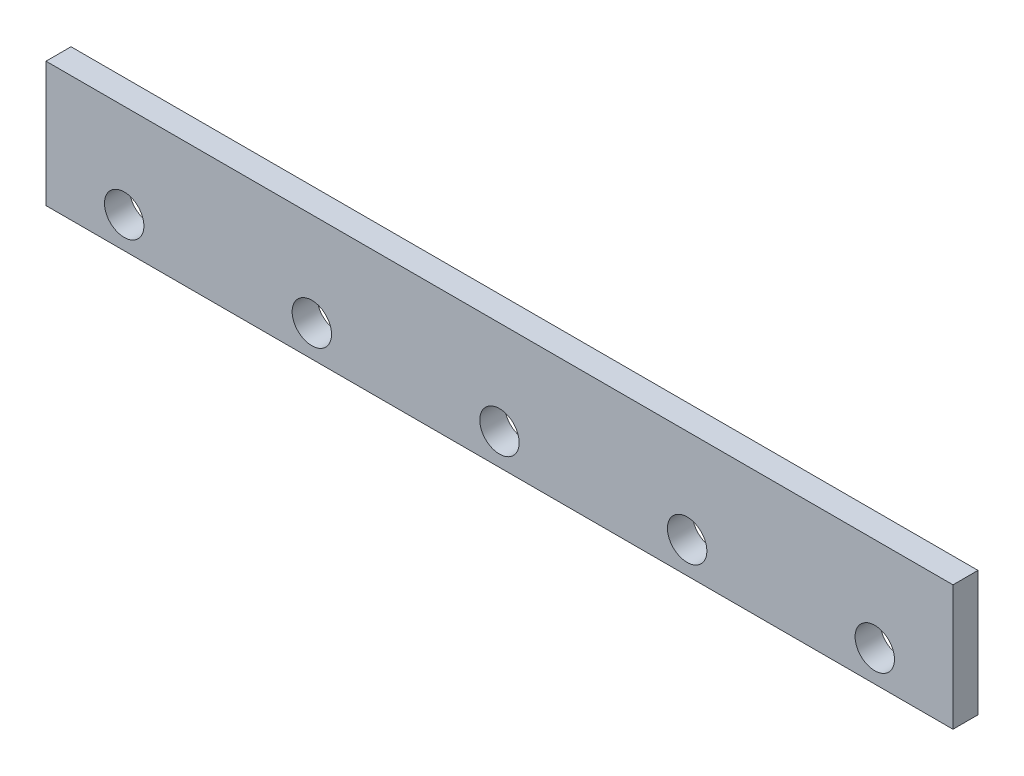
ISO-10303-21;
HEADER;
FILE_DESCRIPTION(('STEP AP214'),'2;1');
FILE_NAME('part.step','',(''),(''),'','','');
FILE_SCHEMA(('AUTOMOTIVE_DESIGN { 1 0 10303 214 1 1 1 1 }'));
ENDSEC;
DATA;
#1=APPLICATION_CONTEXT('core data for automotive mechanical design processes');
#2=APPLICATION_PROTOCOL_DEFINITION('international standard','automotive_design',2000,#1);
#3=PRODUCT_CONTEXT('',#1,'mechanical');
#4=PRODUCT('Part','Part','',(#3));
#5=PRODUCT_RELATED_PRODUCT_CATEGORY('part','',(#4));
#6=PRODUCT_DEFINITION_FORMATION('','',#4);
#7=PRODUCT_DEFINITION_CONTEXT('part definition',#1,'design');
#8=PRODUCT_DEFINITION('design','',#6,#7);
#9=PRODUCT_DEFINITION_SHAPE('','',#8);
#10=(LENGTH_UNIT() NAMED_UNIT(*) SI_UNIT(.MILLI.,.METRE.));
#11=(NAMED_UNIT(*) PLANE_ANGLE_UNIT() SI_UNIT($,.RADIAN.));
#12=(NAMED_UNIT(*) SI_UNIT($,.STERADIAN.) SOLID_ANGLE_UNIT());
#13=UNCERTAINTY_MEASURE_WITH_UNIT(LENGTH_MEASURE(1.E-05),#10,'distance_accuracy_value','');
#14=(GEOMETRIC_REPRESENTATION_CONTEXT(3) GLOBAL_UNCERTAINTY_ASSIGNED_CONTEXT((#13)) GLOBAL_UNIT_ASSIGNED_CONTEXT((#10,
#11,#12)) REPRESENTATION_CONTEXT('',''));
#15=CARTESIAN_POINT('',(0.,0.,0.));
#16=DIRECTION('',(0.,0.,1.));
#17=DIRECTION('',(1.,0.,0.));
#18=AXIS2_PLACEMENT_3D('',#15,#16,#17);
#19=CARTESIAN_POINT('',(290.,40.,16.));
#20=DIRECTION('',(-1.,0.,0.));
#21=DIRECTION('',(0.,0.,1.));
#22=AXIS2_PLACEMENT_3D('',#19,#20,#21);
#23=PLANE('',#22);
#24=DIRECTION('',(0.,1.,0.));
#25=VECTOR('',#24,1.);
#26=CARTESIAN_POINT('',(290.,40.,0.));
#27=LINE('',#26,#25);
#28=CARTESIAN_POINT('',(290.,-40.,0.));
#29=VERTEX_POINT('',#28);
#30=CARTESIAN_POINT('',(290.,40.,0.));
#31=VERTEX_POINT('',#30);
#32=EDGE_CURVE('E102',#29,#31,#27,.T.);
#33=ORIENTED_EDGE('',*,*,#32,.T.);
#34=DIRECTION('',(0.,0.,-1.));
#35=VECTOR('',#34,1.);
#36=CARTESIAN_POINT('',(290.,40.,16.));
#37=LINE('',#36,#35);
#38=CARTESIAN_POINT('',(290.,40.,16.));
#39=VERTEX_POINT('',#38);
#40=EDGE_CURVE('E11',#39,#31,#37,.T.);
#41=ORIENTED_EDGE('',*,*,#40,.F.);
#42=DIRECTION('',(0.,1.,0.));
#43=VECTOR('',#42,1.);
#44=CARTESIAN_POINT('',(290.,40.,16.));
#45=LINE('',#44,#43);
#46=CARTESIAN_POINT('',(290.,-40.,16.));
#47=VERTEX_POINT('',#46);
#48=EDGE_CURVE('E95',#47,#39,#45,.T.);
#49=ORIENTED_EDGE('',*,*,#48,.F.);
#50=DIRECTION('',(0.,0.,-1.));
#51=VECTOR('',#50,1.);
#52=CARTESIAN_POINT('',(290.,-40.,16.));
#53=LINE('',#52,#51);
#54=EDGE_CURVE('E103',#47,#29,#53,.T.);
#55=ORIENTED_EDGE('',*,*,#54,.T.);
#56=EDGE_LOOP('',(#33,#41,#49,#55));
#57=FACE_BOUND('',#56,.T.);
#58=ADVANCED_FACE('F39',(#57),#23,.F.);
#59=CARTESIAN_POINT('',(-290.,40.,16.));
#60=DIRECTION('',(0.,-1.,0.));
#61=DIRECTION('',(0.,0.,-1.));
#62=AXIS2_PLACEMENT_3D('',#59,#60,#61);
#63=PLANE('',#62);
#64=DIRECTION('',(-1.,0.,0.));
#65=VECTOR('',#64,1.);
#66=CARTESIAN_POINT('',(-290.,40.,0.));
#67=LINE('',#66,#65);
#68=CARTESIAN_POINT('',(-290.,40.,0.));
#69=VERTEX_POINT('',#68);
#70=EDGE_CURVE('E98',#31,#69,#67,.T.);
#71=ORIENTED_EDGE('',*,*,#70,.T.);
#72=DIRECTION('',(0.,0.,-1.));
#73=VECTOR('',#72,1.);
#74=CARTESIAN_POINT('',(-290.,40.,16.));
#75=LINE('',#74,#73);
#76=CARTESIAN_POINT('',(-290.,40.,16.));
#77=VERTEX_POINT('',#76);
#78=EDGE_CURVE('E48',#77,#69,#75,.T.);
#79=ORIENTED_EDGE('',*,*,#78,.F.);
#80=DIRECTION('',(-1.,0.,0.));
#81=VECTOR('',#80,1.);
#82=CARTESIAN_POINT('',(-290.,40.,16.));
#83=LINE('',#82,#81);
#84=EDGE_CURVE('E90',#39,#77,#83,.T.);
#85=ORIENTED_EDGE('',*,*,#84,.F.);
#86=ORIENTED_EDGE('',*,*,#40,.T.);
#87=EDGE_LOOP('',(#71,#79,#85,#86));
#88=FACE_BOUND('',#87,.T.);
#89=ADVANCED_FACE('F94',(#88),#63,.F.);
#90=CARTESIAN_POINT('',(-290.,40.,16.));
#91=DIRECTION('',(1.,0.,0.));
#92=DIRECTION('',(0.,0.,-1.));
#93=AXIS2_PLACEMENT_3D('',#90,#91,#92);
#94=PLANE('',#93);
#95=DIRECTION('',(0.,-1.,0.));
#96=VECTOR('',#95,1.);
#97=CARTESIAN_POINT('',(-290.,40.,0.));
#98=LINE('',#97,#96);
#99=CARTESIAN_POINT('',(-290.,-40.,0.));
#100=VERTEX_POINT('',#99);
#101=EDGE_CURVE('E72',#69,#100,#98,.T.);
#102=ORIENTED_EDGE('',*,*,#101,.T.);
#103=DIRECTION('',(0.,0.,-1.));
#104=VECTOR('',#103,1.);
#105=CARTESIAN_POINT('',(-290.,-40.,16.));
#106=LINE('',#105,#104);
#107=CARTESIAN_POINT('',(-290.,-40.,16.));
#108=VERTEX_POINT('',#107);
#109=EDGE_CURVE('E97',#108,#100,#106,.T.);
#110=ORIENTED_EDGE('',*,*,#109,.F.);
#111=DIRECTION('',(0.,-1.,0.));
#112=VECTOR('',#111,1.);
#113=CARTESIAN_POINT('',(-290.,40.,16.));
#114=LINE('',#113,#112);
#115=EDGE_CURVE('E89',#77,#108,#114,.T.);
#116=ORIENTED_EDGE('',*,*,#115,.F.);
#117=ORIENTED_EDGE('',*,*,#78,.T.);
#118=EDGE_LOOP('',(#102,#110,#116,#117));
#119=FACE_BOUND('',#118,.T.);
#120=ADVANCED_FACE('F100',(#119),#94,.F.);
#121=CARTESIAN_POINT('',(-290.,-40.,16.));
#122=DIRECTION('',(0.,1.,0.));
#123=DIRECTION('',(0.,0.,1.));
#124=AXIS2_PLACEMENT_3D('',#121,#122,#123);
#125=PLANE('',#124);
#126=DIRECTION('',(1.,0.,0.));
#127=VECTOR('',#126,1.);
#128=CARTESIAN_POINT('',(-290.,-40.,0.));
#129=LINE('',#128,#127);
#130=EDGE_CURVE('E78',#100,#29,#129,.T.);
#131=ORIENTED_EDGE('',*,*,#130,.T.);
#132=ORIENTED_EDGE('',*,*,#54,.F.);
#133=DIRECTION('',(1.,0.,0.));
#134=VECTOR('',#133,1.);
#135=CARTESIAN_POINT('',(-290.,-40.,16.));
#136=LINE('',#135,#134);
#137=EDGE_CURVE('E60',#108,#47,#136,.T.);
#138=ORIENTED_EDGE('',*,*,#137,.F.);
#139=ORIENTED_EDGE('',*,*,#109,.T.);
#140=EDGE_LOOP('',(#131,#132,#138,#139));
#141=FACE_BOUND('',#140,.T.);
#142=ADVANCED_FACE('F159',(#141),#125,.F.);
#143=CARTESIAN_POINT('',(0.,0.,16.));
#144=DIRECTION('',(0.,0.,1.));
#145=DIRECTION('',(1.,0.,0.));
#146=AXIS2_PLACEMENT_3D('',#143,#144,#145);
#147=PLANE('',#146);
#148=CARTESIAN_POINT('',(-240.,-20.,16.));
#149=DIRECTION('',(0.,0.,1.));
#150=DIRECTION('',(1.,0.,0.));
#151=AXIS2_PLACEMENT_3D('',#148,#149,#150);
#152=CIRCLE('',#151,12.6);
#153=CARTESIAN_POINT('',(-227.4,-20.,16.));
#154=VERTEX_POINT('',#153);
#155=EDGE_CURVE('E120',#154,#154,#152,.T.);
#156=ORIENTED_EDGE('',*,*,#155,.F.);
#157=EDGE_LOOP('',(#156));
#158=FACE_BOUND('',#157,.T.);
#159=CARTESIAN_POINT('',(-120.,-20.,16.));
#160=DIRECTION('',(0.,0.,1.));
#161=DIRECTION('',(1.,0.,0.));
#162=AXIS2_PLACEMENT_3D('',#159,#160,#161);
#163=CIRCLE('',#162,12.6);
#164=CARTESIAN_POINT('',(-107.4,-20.,16.));
#165=VERTEX_POINT('',#164);
#166=EDGE_CURVE('E236',#165,#165,#163,.T.);
#167=ORIENTED_EDGE('',*,*,#166,.F.);
#168=EDGE_LOOP('',(#167));
#169=FACE_BOUND('',#168,.T.);
#170=CARTESIAN_POINT('',(1.11022302462516E-13,-20.,16.));
#171=DIRECTION('',(0.,0.,1.));
#172=DIRECTION('',(1.,0.,0.));
#173=AXIS2_PLACEMENT_3D('',#170,#171,#172);
#174=CIRCLE('',#173,12.6);
#175=CARTESIAN_POINT('',(12.6000000000001,-20.,16.));
#176=VERTEX_POINT('',#175);
#177=EDGE_CURVE('E228',#176,#176,#174,.T.);
#178=ORIENTED_EDGE('',*,*,#177,.F.);
#179=EDGE_LOOP('',(#178));
#180=FACE_BOUND('',#179,.T.);
#181=CARTESIAN_POINT('',(120.,-20.,16.));
#182=DIRECTION('',(0.,0.,1.));
#183=DIRECTION('',(1.,0.,0.));
#184=AXIS2_PLACEMENT_3D('',#181,#182,#183);
#185=CIRCLE('',#184,12.6);
#186=CARTESIAN_POINT('',(132.6,-20.,16.));
#187=VERTEX_POINT('',#186);
#188=EDGE_CURVE('E240',#187,#187,#185,.T.);
#189=ORIENTED_EDGE('',*,*,#188,.F.);
#190=EDGE_LOOP('',(#189));
#191=FACE_BOUND('',#190,.T.);
#192=CARTESIAN_POINT('',(240.,-20.,16.));
#193=DIRECTION('',(0.,0.,1.));
#194=DIRECTION('',(1.,0.,0.));
#195=AXIS2_PLACEMENT_3D('',#192,#193,#194);
#196=CIRCLE('',#195,12.6);
#197=CARTESIAN_POINT('',(252.6,-20.,16.));
#198=VERTEX_POINT('',#197);
#199=EDGE_CURVE('E245',#198,#198,#196,.T.);
#200=ORIENTED_EDGE('',*,*,#199,.F.);
#201=EDGE_LOOP('',(#200));
#202=FACE_BOUND('',#201,.T.);
#203=ORIENTED_EDGE('',*,*,#48,.T.);
#204=ORIENTED_EDGE('',*,*,#84,.T.);
#205=ORIENTED_EDGE('',*,*,#115,.T.);
#206=ORIENTED_EDGE('',*,*,#137,.T.);
#207=EDGE_LOOP('',(#203,#204,#205,#206));
#208=FACE_BOUND('',#207,.T.);
#209=ADVANCED_FACE('F88',(#158,#169,#180,#191,#202,#208),#147,.T.);
#210=CARTESIAN_POINT('',(0.,0.,0.));
#211=DIRECTION('',(0.,0.,1.));
#212=DIRECTION('',(1.,0.,0.));
#213=AXIS2_PLACEMENT_3D('',#210,#211,#212);
#214=PLANE('',#213);
#215=CARTESIAN_POINT('',(-240.,-20.,0.));
#216=DIRECTION('',(0.,0.,1.));
#217=DIRECTION('',(1.,0.,0.));
#218=AXIS2_PLACEMENT_3D('',#215,#216,#217);
#219=CIRCLE('',#218,12.6);
#220=CARTESIAN_POINT('',(-227.4,-20.,0.));
#221=VERTEX_POINT('',#220);
#222=EDGE_CURVE('E45',#221,#221,#219,.T.);
#223=ORIENTED_EDGE('',*,*,#222,.T.);
#224=EDGE_LOOP('',(#223));
#225=FACE_BOUND('',#224,.T.);
#226=CARTESIAN_POINT('',(-120.,-20.,0.));
#227=DIRECTION('',(0.,0.,1.));
#228=DIRECTION('',(1.,0.,0.));
#229=AXIS2_PLACEMENT_3D('',#226,#227,#228);
#230=CIRCLE('',#229,12.6);
#231=CARTESIAN_POINT('',(-107.4,-20.,0.));
#232=VERTEX_POINT('',#231);
#233=EDGE_CURVE('E125',#232,#232,#230,.T.);
#234=ORIENTED_EDGE('',*,*,#233,.T.);
#235=EDGE_LOOP('',(#234));
#236=FACE_BOUND('',#235,.T.);
#237=CARTESIAN_POINT('',(1.11022302462516E-13,-20.,0.));
#238=DIRECTION('',(0.,0.,1.));
#239=DIRECTION('',(1.,0.,0.));
#240=AXIS2_PLACEMENT_3D('',#237,#238,#239);
#241=CIRCLE('',#240,12.6);
#242=CARTESIAN_POINT('',(12.6000000000001,-20.,0.));
#243=VERTEX_POINT('',#242);
#244=EDGE_CURVE('E119',#243,#243,#241,.T.);
#245=ORIENTED_EDGE('',*,*,#244,.T.);
#246=EDGE_LOOP('',(#245));
#247=FACE_BOUND('',#246,.T.);
#248=CARTESIAN_POINT('',(120.,-20.,0.));
#249=DIRECTION('',(0.,0.,1.));
#250=DIRECTION('',(1.,0.,0.));
#251=AXIS2_PLACEMENT_3D('',#248,#249,#250);
#252=CIRCLE('',#251,12.6);
#253=CARTESIAN_POINT('',(132.6,-20.,0.));
#254=VERTEX_POINT('',#253);
#255=EDGE_CURVE('E116',#254,#254,#252,.T.);
#256=ORIENTED_EDGE('',*,*,#255,.T.);
#257=EDGE_LOOP('',(#256));
#258=FACE_BOUND('',#257,.T.);
#259=CARTESIAN_POINT('',(240.,-20.,0.));
#260=DIRECTION('',(0.,0.,1.));
#261=DIRECTION('',(1.,0.,0.));
#262=AXIS2_PLACEMENT_3D('',#259,#260,#261);
#263=CIRCLE('',#262,12.6);
#264=CARTESIAN_POINT('',(252.6,-20.,0.));
#265=VERTEX_POINT('',#264);
#266=EDGE_CURVE('E113',#265,#265,#263,.T.);
#267=ORIENTED_EDGE('',*,*,#266,.T.);
#268=EDGE_LOOP('',(#267));
#269=FACE_BOUND('',#268,.T.);
#270=ORIENTED_EDGE('',*,*,#32,.F.);
#271=ORIENTED_EDGE('',*,*,#130,.F.);
#272=ORIENTED_EDGE('',*,*,#101,.F.);
#273=ORIENTED_EDGE('',*,*,#70,.F.);
#274=EDGE_LOOP('',(#270,#271,#272,#273));
#275=FACE_BOUND('',#274,.T.);
#276=ADVANCED_FACE('F126',(#225,#236,#247,#258,#269,#275),#214,.F.);
#277=CARTESIAN_POINT('',(240.,-20.,-10.));
#278=DIRECTION('',(0.,0.,1.));
#279=DIRECTION('',(1.,0.,0.));
#280=AXIS2_PLACEMENT_3D('',#277,#278,#279);
#281=CYLINDRICAL_SURFACE('',#280,12.6);
#282=ORIENTED_EDGE('',*,*,#199,.T.);
#283=EDGE_LOOP('',(#282));
#284=FACE_BOUND('',#283,.T.);
#285=ORIENTED_EDGE('',*,*,#266,.F.);
#286=EDGE_LOOP('',(#285));
#287=FACE_BOUND('',#286,.T.);
#288=ADVANCED_FACE('F151',(#284,#287),#281,.F.);
#289=CARTESIAN_POINT('',(120.,-20.,-10.));
#290=DIRECTION('',(0.,0.,1.));
#291=DIRECTION('',(1.,0.,0.));
#292=AXIS2_PLACEMENT_3D('',#289,#290,#291);
#293=CYLINDRICAL_SURFACE('',#292,12.6);
#294=ORIENTED_EDGE('',*,*,#188,.T.);
#295=EDGE_LOOP('',(#294));
#296=FACE_BOUND('',#295,.T.);
#297=ORIENTED_EDGE('',*,*,#255,.F.);
#298=EDGE_LOOP('',(#297));
#299=FACE_BOUND('',#298,.T.);
#300=ADVANCED_FACE('F160',(#296,#299),#293,.F.);
#301=CARTESIAN_POINT('',(1.11022302462516E-13,-20.,-10.));
#302=DIRECTION('',(0.,0.,1.));
#303=DIRECTION('',(1.,0.,0.));
#304=AXIS2_PLACEMENT_3D('',#301,#302,#303);
#305=CYLINDRICAL_SURFACE('',#304,12.6);
#306=ORIENTED_EDGE('',*,*,#177,.T.);
#307=EDGE_LOOP('',(#306));
#308=FACE_BOUND('',#307,.T.);
#309=ORIENTED_EDGE('',*,*,#244,.F.);
#310=EDGE_LOOP('',(#309));
#311=FACE_BOUND('',#310,.T.);
#312=ADVANCED_FACE('F137',(#308,#311),#305,.F.);
#313=CARTESIAN_POINT('',(-120.,-20.,-10.));
#314=DIRECTION('',(0.,0.,1.));
#315=DIRECTION('',(1.,0.,0.));
#316=AXIS2_PLACEMENT_3D('',#313,#314,#315);
#317=CYLINDRICAL_SURFACE('',#316,12.6);
#318=ORIENTED_EDGE('',*,*,#166,.T.);
#319=EDGE_LOOP('',(#318));
#320=FACE_BOUND('',#319,.T.);
#321=ORIENTED_EDGE('',*,*,#233,.F.);
#322=EDGE_LOOP('',(#321));
#323=FACE_BOUND('',#322,.T.);
#324=ADVANCED_FACE('F133',(#320,#323),#317,.F.);
#325=CARTESIAN_POINT('',(-240.,-20.,-10.));
#326=DIRECTION('',(0.,0.,1.));
#327=DIRECTION('',(1.,0.,0.));
#328=AXIS2_PLACEMENT_3D('',#325,#326,#327);
#329=CYLINDRICAL_SURFACE('',#328,12.6);
#330=ORIENTED_EDGE('',*,*,#155,.T.);
#331=EDGE_LOOP('',(#330));
#332=FACE_BOUND('',#331,.T.);
#333=ORIENTED_EDGE('',*,*,#222,.F.);
#334=EDGE_LOOP('',(#333));
#335=FACE_BOUND('',#334,.T.);
#336=ADVANCED_FACE('F131',(#332,#335),#329,.F.);
#337=CLOSED_SHELL('',(#58,#89,#120,#142,#209,#276,#288,#300,#312,#324,#336));
#338=MANIFOLD_SOLID_BREP('B2',#337);
#339=ADVANCED_BREP_SHAPE_REPRESENTATION('',(#18,#338),#14);
#340=SHAPE_DEFINITION_REPRESENTATION(#9,#339);
ENDSEC;
END-ISO-10303-21;
